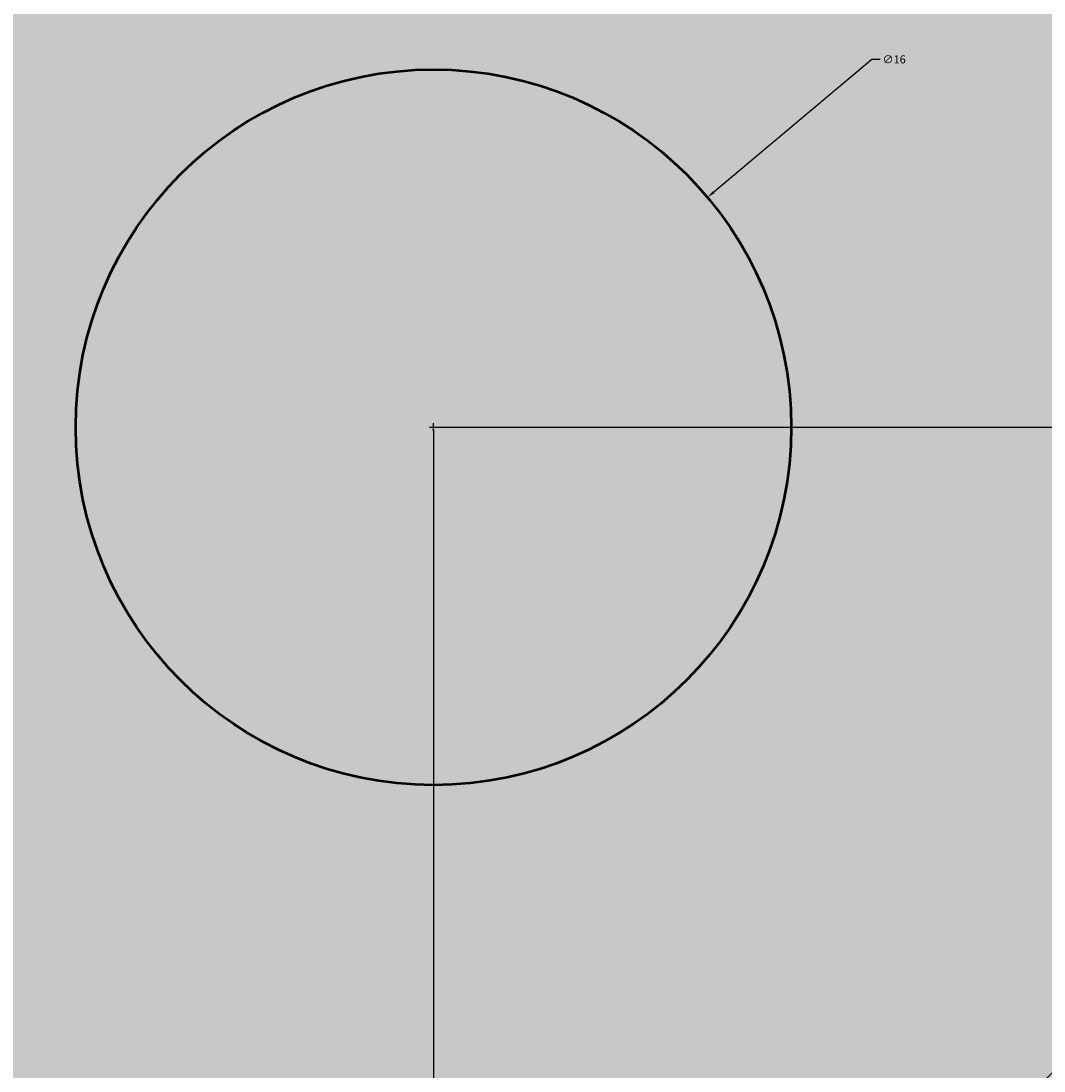
# Model space of a CAD drawing. Units: inches. Extents: x 114 to 236, y -51 to 115.
# Tile 11 of 14: x 166 to 189, y 65 to 88. Entities that reach past the tile are written whole.
import ezdxf

# ---------------------------------------------------------------- set-up
doc = ezdxf.new("R2010")
doc.units = ezdxf.units.IN
doc.header["$MEASUREMENT"] = 0
doc.linetypes.add('CENTER', pattern=[50.8, 31.75, -6.35, 6.35, -6.35])
for name, color, linetype, lineweight in [('M-CNTR', 7, 'CENTER', 18), ('M-DIMS', 2, 'Continuous', 18), ('M-OUTL', 7, 'Continuous', 50)]:
    doc.layers.add(name, color=color, linetype=linetype, lineweight=lineweight)
doc.layers.add('M-HATC', color=7, linetype='Continuous', lineweight=18, true_color=0xffffff)
doc.styles.get("Standard").update_dxf_attribs({"font": 'arial.ttf'})
doc.dimstyles.get("Standard").update_dxf_attribs({"dimtxt": 0.18, "dimasz": 0.18, "dimexe": 0.18, "dimexo": 0.0625, "dimgap": 0.09, "dimtad": 0, "dimtih": 1, "dimtoh": 1, "dimdec": 4, "dimzin": 0, "dimdsep": 46, "dimtxsty": 'Standard', "dimcen": 0.09, "dimadec": 0, "dimazin": 0, "dimtfac": 1, "dimtdec": 4, "dimtofl": 0, "dimtmove": 0, "dimatfit": 3, "dimfxl": 1, "dimtolj": 1, "dimtzin": 0, "dimarcsym": 0})

# ---------------------------------------------------------------- blocks, each defined once
blk = doc.blocks.new('*D3')
at = {"layer": 'Defpoints', "color": 0, "transparency": 16777216}
for p in [(230.229, 115.287), (120.229, 9.307), (230.229, 9.307)]:
    blk.add_point(p, dxfattribs=at)
at = {"layer": 'M-DIMS', "color": 0, "lineweight": -2, "transparency": 16777216}
for p, q in [((120.229, 9.37), (120.229, 115.467)), ((120.409, 115.287), (174.949, 115.287)), ((230.049, 115.287), (175.509, 115.287)), ((230.229, 9.37), (230.229, 115.467))]:
    blk.add_line(p, q, dxfattribs=at)
at = {"layer": 'M-DIMS', "color": 0, "transparency": 16777216}
for points in [[(120.409, 115.317), (120.409, 115.257), (120.229, 115.287)], [(230.049, 115.317), (230.049, 115.257), (230.229, 115.287)]]:
    blk.add_solid(points, dxfattribs=at)
at = {"layer": 'M-DIMS', "color": 0, "transparency": 16777216, "insert": (175.229, 115.287), "char_height": 0.18, "attachment_point": 5}
blk.add_mtext('\\A1;110', dxfattribs=at)
blk = doc.blocks.new('*D4')
at = {"layer": 'Defpoints', "color": 0, "transparency": 16777216}
for p in [(114.249, 109.307), (175.229, 109.307), (135.229, -5.693)]:
    blk.add_point(p, dxfattribs=at)
at = {"layer": 'M-DIMS', "color": 0, "lineweight": -2, "transparency": 16777216}
for p, q in [((175.166, 109.307), (114.069, 109.307)), ((114.249, 109.127), (114.249, 51.989)), ((114.249, -5.513), (114.249, 51.625)), ((135.166, -5.693), (114.069, -5.693))]:
    blk.add_line(p, q, dxfattribs=at)
at = {"layer": 'M-DIMS', "color": 0, "transparency": 16777216}
for points in [[(114.219, 109.127), (114.279, 109.127), (114.249, 109.307)], [(114.219, -5.513), (114.279, -5.513), (114.249, -5.693)]]:
    blk.add_solid(points, dxfattribs=at)
at = {"layer": 'M-DIMS', "color": 0, "transparency": 16777216, "insert": (114.249, 51.807), "char_height": 0.18, "attachment_point": 5}
blk.add_mtext('\\A1;115', dxfattribs=at)
blk = doc.blocks.new('*D5')
at = {"layer": 'Defpoints', "color": 0, "transparency": 16777216}
for p in [(175.229, 79.307), (135.229, 9.307), (175.229, -11.673)]:
    blk.add_point(p, dxfattribs=at)
at = {"layer": 'M-DIMS', "color": 0, "lineweight": -2, "transparency": 16777216}
for p, q in [((175.229, 79.245), (175.229, -11.853)), ((135.229, 9.245), (135.229, -11.853)), ((135.409, -11.673), (155.006, -11.673)), ((175.049, -11.673), (155.451, -11.673))]:
    blk.add_line(p, q, dxfattribs=at)
at = {"layer": 'M-DIMS', "color": 0, "transparency": 16777216}
for points in [[(135.409, -11.643), (135.409, -11.703), (135.229, -11.673)], [(175.049, -11.643), (175.049, -11.703), (175.229, -11.673)]]:
    blk.add_solid(points, dxfattribs=at)
at = {"layer": 'M-DIMS', "color": 0, "transparency": 16777216, "insert": (155.229, -11.673), "char_height": 0.18, "attachment_point": 5}
blk.add_mtext('\\A1;40', dxfattribs=at)
blk = doc.blocks.new('*D6')
at = {"layer": 'Defpoints', "color": 0, "transparency": 16777216}
for p in [(175.229, 79.307), (215.229, 9.307), (215.229, -11.673)]:
    blk.add_point(p, dxfattribs=at)
at = {"layer": 'M-DIMS', "color": 0, "lineweight": -2, "transparency": 16777216}
for p, q in [((175.229, 79.245), (175.229, -11.853)), ((215.229, 9.245), (215.229, -11.853)), ((175.409, -11.673), (195.006, -11.673)), ((215.049, -11.673), (195.451, -11.673))]:
    blk.add_line(p, q, dxfattribs=at)
at = {"layer": 'M-DIMS', "color": 0, "transparency": 16777216}
for points in [[(175.409, -11.643), (175.409, -11.703), (175.229, -11.673)], [(215.049, -11.643), (215.049, -11.703), (215.229, -11.673)]]:
    blk.add_solid(points, dxfattribs=at)
at = {"layer": 'M-DIMS', "color": 0, "transparency": 16777216, "insert": (195.229, -11.673), "char_height": 0.18, "attachment_point": 5}
blk.add_mtext('\\A1;40', dxfattribs=at)
blk = doc.blocks.new('*D7')
at = {"layer": 'Defpoints', "color": 0, "transparency": 16777216}
for p in [(175.229, 79.307), (236.209, 79.307), (215.229, 9.307)]:
    blk.add_point(p, dxfattribs=at)
at = {"layer": 'M-DIMS', "color": 0, "lineweight": -2, "transparency": 16777216}
for p, q in [((175.291, 79.307), (236.389, 79.307)), ((236.209, 79.127), (236.209, 44.489)), ((236.209, 9.487), (236.209, 44.125)), ((215.291, 9.307), (236.389, 9.307))]:
    blk.add_line(p, q, dxfattribs=at)
at = {"layer": 'M-DIMS', "color": 0, "transparency": 16777216}
for points in [[(236.179, 79.127), (236.239, 79.127), (236.209, 79.307)], [(236.179, 9.487), (236.239, 9.487), (236.209, 9.307)]]:
    blk.add_solid(points, dxfattribs=at)
at = {"layer": 'M-DIMS', "color": 0, "transparency": 16777216, "insert": (236.209, 44.307), "char_height": 0.18, "attachment_point": 5}
blk.add_mtext('\\A1;70', dxfattribs=at)
blk = doc.blocks.new('*D8')
at = {"layer": 'Defpoints', "color": 0, "transparency": 16777216}
for p in [(197.149, 99.789), (153.308, 58.825)]:
    blk.add_point(p, dxfattribs=at)
at = {"layer": 'M-DIMS', "color": 0, "lineweight": -2, "transparency": 16777216}
for p, q in [((210.301, 112.078), (197.28, 99.912)), ((210.481, 112.078), (210.301, 112.078)), ((175.229, 79.217), (175.229, 79.397)), ((175.139, 79.307), (175.319, 79.307))]:
    blk.add_line(p, q, dxfattribs=at)
at = {"layer": 'M-DIMS', "color": 0, "transparency": 16777216}
blk.add_solid([(197.26, 99.934), (197.301, 99.89), (197.149, 99.789)], dxfattribs=at)
at = {"layer": 'M-DIMS', "color": 0, "transparency": 16777216, "insert": (210.797, 112.078), "char_height": 0.18, "attachment_point": 5}
blk.add_mtext('\\A1;∅60', dxfattribs=at)
blk = doc.blocks.new('*D9')
at = {"layer": 'Defpoints', "color": 0, "transparency": 16777216}
for p in [(157.908, 89.307), (192.549, 69.307)]:
    blk.add_point(p, dxfattribs=at)
at = {"layer": 'M-DIMS', "color": 0, "lineweight": -2, "transparency": 16777216}
for p, q in [((147.336, 95.307), (147.516, 95.307)), ((147.516, 95.307), (157.752, 89.397)), ((175.229, 79.217), (175.229, 79.397)), ((175.139, 79.307), (175.319, 79.307))]:
    blk.add_line(p, q, dxfattribs=at)
at = {"layer": 'M-DIMS', "color": 0, "transparency": 16777216}
blk.add_solid([(157.767, 89.423), (157.737, 89.371), (157.908, 89.307)], dxfattribs=at)
at = {"layer": 'M-DIMS', "color": 0, "transparency": 16777216, "insert": (147.019, 95.307), "char_height": 0.18, "attachment_point": 5}
blk.add_mtext('\\A1;∅40', dxfattribs=at)
blk = doc.blocks.new('*D10')
at = {"layer": 'Defpoints', "color": 0, "transparency": 16777216}
for p in [(181.358, 84.448), (169.099, 74.166)]:
    blk.add_point(p, dxfattribs=at)
at = {"layer": 'M-DIMS', "color": 0, "lineweight": -2, "transparency": 16777216}
for p, q in [((185.036, 87.533), (181.496, 84.564)), ((185.216, 87.533), (185.036, 87.533)), ((175.229, 79.217), (175.229, 79.397)), ((175.139, 79.307), (175.319, 79.307))]:
    blk.add_line(p, q, dxfattribs=at)
at = {"layer": 'M-DIMS', "color": 0, "transparency": 16777216}
blk.add_solid([(181.477, 84.587), (181.515, 84.541), (181.358, 84.448)], dxfattribs=at)
at = {"layer": 'M-DIMS', "color": 0, "transparency": 16777216, "insert": (185.532, 87.533), "char_height": 0.18, "attachment_point": 5}
blk.add_mtext('\\A1;∅16', dxfattribs=at)

msp = doc.modelspace()

# ---------------------------------------------------------------- hatches: boundary and pattern name
at = {"layer": 'M-HATC'}
h = msp.add_hatch(color=256, dxfattribs=at)
h.set_gradient(color1=(19, 155, 72), color2=(255, 255, 0), tint=1, name='HEMISPHERICAL')
h.paths.add_polyline_path([(147.853, 91.577), (146.105, 86.505, 0.060651), (145.229, 79.307, 1), (205.229, 79.307, 0.060651), (204.352, 86.505), (202.605, 91.577, 0.647643)])
h.paths.add_polyline_path([(180.229, 99.307, -0.031342), (180.189, 98.682, -0.27393), (194.604, 84.268, -0.451416), (200.229, 79.307, -0.451416), (194.604, 74.346, -0.27393), (180.189, 59.932, -0.031342), (180.229, 59.307, -1), (170.229, 59.307, -0.031342), (170.268, 59.932, -0.27393), (155.854, 74.346, -0.451416), (150.229, 79.307, -0.451416), (155.854, 84.268, -0.27393), (170.268, 98.682, -0.031342), (170.229, 99.307, -1)], flags=16)
h.paths.add_polyline_path([(183.229, 79.307, -1), (167.229, 79.307, -1)], flags=0)
h.paths.add_polyline_path([(155.854, 84.268, -0.377964), (160.229, 79.307, -0.377964), (155.854, 74.346, 0.27393), (170.268, 59.932, -0.881917), (180.189, 59.932, 0.27393), (194.604, 74.346, -0.377964), (190.229, 79.307, -0.377964), (194.604, 84.268, 0.27393), (180.189, 98.682, -0.881917), (170.268, 98.682, 0.27393)], flags=0)
msp.add_hatch(color=256, dxfattribs=at).paths.add_polyline_path([(167.229, 79.307, 1), (183.229, 79.307, 1)])
h = msp.add_hatch(color=256, dxfattribs=at)
h.set_gradient(color1=(242, 103, 34), color2=(255, 255, 0), tint=1, name='INVSPHERICAL')
h.paths.add_polyline_path([(145.229, 79.307, -0.060651), (146.105, 86.505), (121.823, 16.038, -0.790743), (150.229, 9.307, -0.236068), (144.229, -2.693, -0.14094), (175.229, 9.098, -0.14094), (206.229, -2.693, -0.236068), (200.229, 9.307, -0.790743), (228.634, 16.038), (204.352, 86.505, -0.060651), (205.229, 79.307, -1)])

# ---------------------------------------------------------------- linework, layer by layer
at = {"layer": 'M-CNTR'}
msp.add_circle((175.229, 79.307), 20, dxfattribs=at)
at = {"layer": 'M-OUTL'}
for radius in [30, 8]:
    msp.add_circle((175.229, 79.307), radius, dxfattribs=at)

# ---------------------------------------------------------------- dimensions: what is measured, and where the dimension line sits
at = {"layer": 'M-DIMS'}
for base, p1, p2, picture, middle in [((230.229, 115.287), (120.229, 9.307), (230.229, 9.307), '*D3', (175.229, 115.287)), ((175.229, -11.673), (135.229, 9.307), (175.229, 79.307), '*D5', (155.229, -11.673)), ((215.229, -11.673), (175.229, 79.307), (215.229, 9.307), '*D6', (195.229, -11.673))]:
    dim = msp.add_linear_dim(base=base, p1=p1, p2=p2, dimstyle='Standard', override={"dimdec": 0, "dimlfac": 1, "dimrnd": 0, "dimzin": 0, "dimdsep": 46, "dimlunit": 2}, dxfattribs=at)
    dim.commit()
    dim.dimension.update_dxf_attribs({"geometry": picture, "text_midpoint": middle})
for p1, p2, picture, middle in [((153.308, 58.825), (197.149, 99.789), '*D8', (210.797, 112.078)), ((192.549, 69.307), (157.908, 89.307), '*D9', (147.019, 95.307)), ((169.099, 74.166), (181.358, 84.448), '*D10', (185.532, 87.533))]:
    dim = msp.add_diameter_dim_2p(p1=p1, p2=p2, dimstyle='Standard', override={"dimdec": 0, "dimlfac": 1, "dimrnd": 0, "dimzin": 0, "dimdsep": 46, "dimlunit": 2}, dxfattribs=at)
    dim.commit()
    dim.dimension.update_dxf_attribs({"geometry": picture, "text_midpoint": middle, "dimtype": 163})
for base, p1, p2, picture, middle in [((114.249, 109.307), (135.229, -5.693), (175.229, 109.307), '*D4', (114.249, 51.807)), ((236.209, 79.307), (215.229, 9.307), (175.229, 79.307), '*D7', (236.209, 44.307))]:
    dim = msp.add_linear_dim(base=base, p1=p1, p2=p2, angle=90, dimstyle='Standard', override={"dimdec": 0, "dimlfac": 1, "dimrnd": 0, "dimzin": 0, "dimdsep": 46, "dimlunit": 2}, dxfattribs=at)
    dim.commit()
    dim.dimension.update_dxf_attribs({"geometry": picture, "text_midpoint": middle})

doc.saveas('drawing.dxf')
